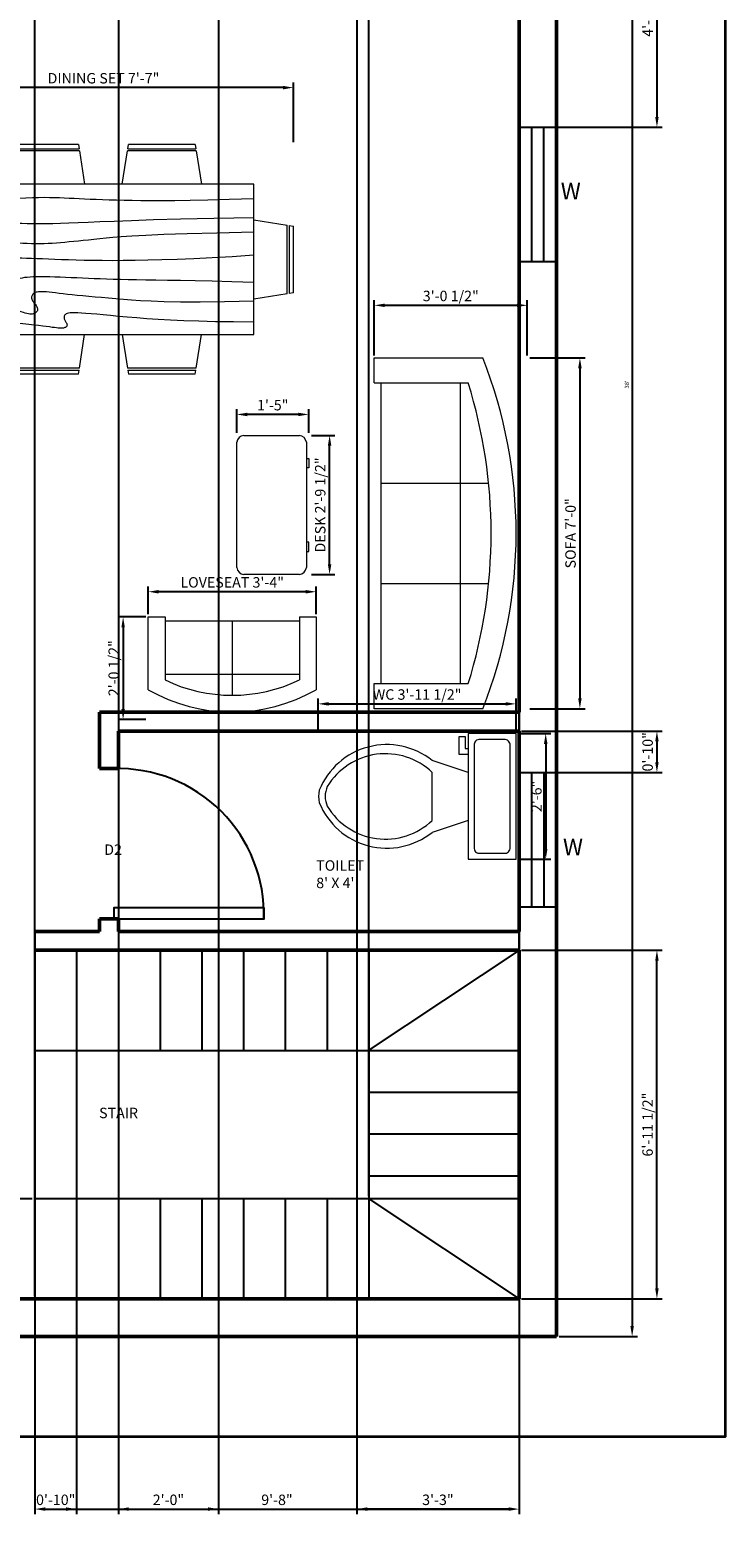
# Model space of a CAD drawing. Units: inches. Extents: x 216 to 622, y 47 to 588.
# Tile 2 of 3: x 455 to 622, y 48 to 403. Entities that reach past the tile are written whole.
import ezdxf

# ---------------------------------------------------------------- set-up
doc = ezdxf.new("R2010")
doc.units = ezdxf.units.IN
for name, color, linetype, lineweight in [('A-ANNO-TTLB', 7, 'Continuous', 35), ('A-AREA-IDEN', 7, 'Continuous', 18), ('A-DOOR', 3, 'Continuous', 25), ('A-FLOR-FIXT', 9, 'Continuous', 18), ('A-FLOR-STRS', 7, 'Continuous', 25), ('A-FURN', 8, 'Continuous', 18), ('A-GLAZ', 4, 'Continuous', 25), ('A-WALL', 7, 'Continuous', 50), ('Dimensions', 1, 'Continuous', 18), ('Text', 6, 'Continuous', 18)]:
    doc.layers.add(name, color=color, linetype=linetype, lineweight=lineweight)
doc.styles.get("Standard").update_dxf_attribs({"font": 'arial.ttf'})
doc.dimstyles.new('ISO-25', dxfattribs={"dimtxt": 2.5, "dimasz": 2.5, "dimexe": 1.25, "dimexo": 0.625, "dimtad": 1, "dimtxsty": 'Standard', "dimcen": 2.5, "dimadec": 0, "dimazin": 0, "dimtfac": 1, "dimtmove": 0, "dimatfit": 3, "dimfxl": 1, "dimarcsym": 0})

# ---------------------------------------------------------------- blocks, each defined once
blk = doc.blocks.new('Sofa - Roundback Loveseat 5 ft.')
for p, q in [((0, -32.44198), (0, -5.99998)), ((-24, -33.99998), (-24, -11.46958)), ((-23.9998, -13.38178), (23.99986, -13.38178)), ((24.00004, -33.99998), (24.00004, -11.46958)), ((-24, -32.44198), (24.00004, -32.44198))]:
    blk.add_line(p, q)
for points in [[(-24, -33.99998), (-30, -33.99998), (-30, -7.99998)], [(30.00004, -7.99998), (30.00004, -33.99998), (24.00004, -33.99998)]]:
    blk.add_lwpolyline(points)
for centre, radius, start, end in [((0, -60.24998), 60.24998, 60.13715, 119.8628), ((0, -61.38438), 55.38444, 64.32083, 115.6792)]:
    blk.add_arc(centre, radius, start, end)
blk = doc.blocks.new('Desk - 30 x 60 in.')
for p, q in [((-26.999995, 0), (26.999995, 0)), ((-29.999995, -27), (-29.999995, -3)), ((29.999995, -3), (29.999995, -27)), ((26.999995, -30), (-26.999995, -30)), ((-20.000005, -30), (-20.000005, -31)), ((-20.000005, -31), (-16.000005, -31)), ((-16.000005, -31), (-16.000005, -30)), ((15.999995, -31), (15.999995, -30)), ((19.999995, -31), (15.999995, -31)), ((19.999995, -30), (19.999995, -31))]:
    blk.add_line(p, q)
for centre, start, end in [((-26.499995, -3.5), 98.1301, 171.8699), ((26.499995, -3.5), 8.130102, 81.8699), ((-26.499995, -26.5), 188.1301, 261.8699), ((26.499995, -26.5), 278.1301, 351.8699)]:
    blk.add_arc(centre, 3.535534, start, end)
blk = doc.blocks.new('Dining Set - 36 x 72 in.')
for p, q in [((-22.2343, 26.00059), (-23.4847, 17.99762)), ((-22.2304, 26), (-5.7608, 26)), ((-22, 27.5), (-22.1562, 26.50042)), ((-5.8416, 26.5), (-22.1534, 26.5)), ((-22, 27.5), (-6, 27.5)), ((-5.8437, 26.49966), (-6, 27.5)), ((-4.5152, 17.99762), (-5.7655, 25.99926)), ((5.7657, 26.00059), (4.5153, 17.99762)), ((5.7696, 26), (22.2392, 26)), ((6, 27.5), (5.8438, 26.50042)), ((22.1584, 26.5), (5.8466, 26.5)), ((6, 27.5), (22, 27.5)), ((22.1563, 26.49966), (22, 27.5)), ((23.4848, 17.99762), (22.2345, 25.99926)), ((36, 18), (-36, 18)), ((-36, 18), (-36, -18)), ((36, -18), (36, 18)), ((-45.5, 8), (-44.5004, 8.15617)), ((-45.5, 8), (-45.5, -8)), ((-44.5, -8.15843), (-44.5, 8.15338)), ((-44.0006, 8.23428), (-35.9976, 9.48474)), ((-44, 8.23041), (-44, -8.23915)), ((44.0006, 8.23428), (35.9976, 9.48474)), ((44, 8.23041), (44, -8.23915)), ((44.5, -8.15843), (44.5, 8.15338)), ((45.5, 8), (44.5005, 8.15617)), ((45.5, 8), (45.5, -8)), ((-44.4997, -8.15631), (-45.5, -8)), ((-35.9976, -9.48476), (-43.9993, -8.2345)), ((35.9976, -9.48476), (43.9993, -8.2345)), ((44.4997, -8.15631), (45.5, -8)), ((-36, -18), (36, -18)), ((-22.2343, -26.0006), (-23.4847, -17.99762)), ((-4.5152, -17.99762), (-5.7655, -25.99928)), ((5.7657, -26.0006), (4.5153, -17.99762)), ((23.4848, -17.99762), (22.2345, -25.99928)), ((-22.2304, -26), (-5.7608, -26)), ((-22, -27.5), (-22.1562, -26.50044)), ((-5.8416, -26.5), (-22.1534, -26.5)), ((-22, -27.5), (-6, -27.5)), ((-5.8437, -26.49967), (-6, -27.5)), ((5.7696, -26), (22.2392, -26)), ((6, -27.5), (5.8438, -26.50044)), ((22.1584, -26.5), (5.8466, -26.5)), ((6, -27.5), (22, -27.5)), ((22.1563, -26.49967), (22, -27.5))]:
    blk.add_line(p, q)
for points in [[(-36, 15), (-31.1772, 14.97754), (-26.8079, 14.91406), (-22.8538, 14.81543), (-19.276, 14.6875), (-16.0362, 14.53613), (-13.0957, 14.36718), (-10.4159, 14.18652), (-7.9583, 14), (-5.6904, 13.81315), (-3.6035, 13.63021), (-1.6954, 13.45508), (0.0365, 13.29166), (1.5945, 13.14388), (2.9811, 13.01562), (4.1988, 12.9108), (5.25, 12.83333), (6.1393, 12.78613), (6.8802, 12.76823), (7.4883, 12.77767), (7.9792, 12.8125), (8.3685, 12.87077), (8.6719, 12.95052), (8.9049, 13.0498), (9.0833, 13.16666), (9.2205, 13.29899), (9.3216, 13.44401), (9.3895, 13.59879), (9.4271, 13.76041), (9.4373, 13.92594), (9.4232, 14.09245), (9.3875, 14.257), (9.3333, 14.41666), (9.2638, 14.56917), (9.1836, 14.71484), (9.0975, 14.85465), (9.0104, 14.98958), (8.9272, 15.1206), (8.8529, 15.2487), (8.7922, 15.37483), (8.75, 15.5), (8.7305, 15.62467), (8.7344, 15.74739), (8.7617, 15.86621), (8.8125, 15.97916), (8.8867, 16.08431), (8.9844, 16.17968), (9.1055, 16.26334), (9.25, 16.33333), (9.4189, 16.38802), (9.6172, 16.42708), (9.8506, 16.45052), (10.125, 16.45833), (10.4463, 16.45052), (10.8203, 16.42708), (11.2529, 16.38802), (11.75, 16.33333), (12.3184, 16.26318), (12.9694, 16.17838), (13.7151, 16.07991), (14.5677, 15.96875), (15.5395, 15.84586), (16.6426, 15.71224), (17.8893, 15.56884), (19.2917, 15.41666), (20.859, 15.25667), (22.5879, 15.08984), (24.4721, 14.91715), (26.5052, 14.73958), (28.6809, 14.5581), (30.9929, 14.3737), (33.4347, 14.18733), (36, 14)], [(-36, 10), (-28.9766, 10.14274), (-23.1725, 10.20442), (-18.4241, 10.19775), (-14.5677, 10.13541), (-11.4399, 10.03011), (-8.877, 9.89453), (-6.7154, 9.74137), (-4.7917, 9.58333), (-2.9698, 9.43082), (-1.2246, 9.28515), (0.4415, 9.14534), (2.026, 9.01041), (3.5266, 8.87939), (4.9408, 8.7513), (6.266, 8.62516), (7.5, 8.5), (8.6411, 8.37549), (9.6914, 8.2539), (10.6538, 8.13818), (11.5312, 8.03125), (12.3267, 7.93603), (13.043, 7.85547), (13.6831, 7.79248), (14.25, 7.75), (14.7471, 7.7303), (15.1797, 7.73307), (15.5537, 7.75732), (15.875, 7.80208), (16.1494, 7.86637), (16.3828, 7.94922), (16.5811, 8.04964), (16.75, 8.16666), (16.8944, 8.29915), (17.0143, 8.44531), (17.1089, 8.60319), (17.1771, 8.77083), (17.218, 8.94629), (17.2305, 9.1276), (17.2137, 9.31282), (17.1667, 9.5), (17.0895, 9.6875), (16.987, 9.875), (16.8649, 10.0625), (16.7292, 10.25), (16.5856, 10.4375), (16.4401, 10.625), (16.2985, 10.8125), (16.1667, 11), (16.05, 11.18733), (15.9518, 11.3737), (15.8752, 11.5581), (15.8229, 11.73958), (15.798, 11.91715), (15.8034, 12.08984), (15.842, 12.25667), (15.9167, 12.41666), (16.0295, 12.56836), (16.1784, 12.70833), (16.3605, 12.83268), (16.5729, 12.9375), (16.8127, 13.01888), (17.0768, 13.07291), (17.3625, 13.0957), (17.6667, 13.08333), (17.9894, 13.03312), (18.3418, 12.94726), (18.7382, 12.82918), (19.1927, 12.68229), (19.7195, 12.51001), (20.3327, 12.31575), (21.0465, 12.10294), (21.875, 11.875), (22.8357, 11.63354), (23.959, 11.37304), (25.2786, 11.08618), (26.8282, 10.76562), (28.6414, 10.40405), (30.752, 9.99414), (33.1936, 9.52856), (36, 9)], [(-36, 5.5), (-30.7157, 5.3348), (-26.069, 5.20963), (-21.9946, 5.11767), (-18.4271, 5.05208), (-15.3009, 5.00602), (-12.5508, 4.97265), (-10.1112, 4.94515), (-7.9167, 4.91666), (-5.909, 4.88167), (-4.0586, 4.83984), (-2.3429, 4.79215), (-0.7396, 4.73958), (0.7739, 4.6831), (2.22, 4.6237), (3.6213, 4.56233), (5, 4.5), (6.373, 4.43782), (7.7344, 4.3776), (9.0723, 4.32129), (10.375, 4.27083), (11.6309, 4.22819), (12.8281, 4.19531), (13.9551, 4.17415), (15, 4.16666), (15.954, 4.17448), (16.819, 4.19791), (17.6001, 4.23698), (18.3021, 4.29166), (18.9299, 4.36198), (19.4883, 4.44791), (19.9823, 4.54948), (20.4167, 4.66666), (20.7969, 4.79899), (21.1302, 4.94401), (21.4245, 5.09879), (21.6875, 5.26041), (21.9271, 5.42594), (22.1511, 5.59245), (22.3672, 5.757), (22.5834, 5.91666), (22.8065, 6.06868), (23.0404, 6.21093), (23.2879, 6.34147), (23.5521, 6.45833), (23.8358, 6.55957), (24.142, 6.64323), (24.4735, 6.70735), (24.8334, 6.75), (25.2235, 6.76969), (25.642, 6.76692), (26.0858, 6.74267), (26.5521, 6.69791), (27.0379, 6.63362), (27.5404, 6.55078), (28.0565, 6.45036), (28.5834, 6.33333), (29.1242, 6.19987), (29.7071, 6.04687), (30.3661, 5.87044), (31.1354, 5.66666), (32.0493, 5.43164), (33.142, 5.16146), (34.4475, 4.85221), (36, 4.5)], [(-36, -1), (-30.7915, -0.6591), (-26.0195, -0.38216), (-21.6519, -0.16284), (-17.6563, 0.00521), (-14.0005, 0.12833), (-10.6523, 0.21289), (-7.5796, 0.26522), (-4.75, 0.29166), (-2.134, 0.29793), (0.2878, 0.28711), (2.5317, 0.26163), (4.6146, 0.22396), (6.5529, 0.17651), (8.3633, 0.12174), (10.0623, 0.06209), (11.6667, 0), (13.1899, -0.06201), (14.6341, -0.1211), (15.9982, -0.17432), (17.2813, -0.21875), (18.4823, -0.25147), (19.6003, -0.26953), (20.6343, -0.27002), (21.5834, -0.25), (22.4481, -0.20768), (23.2357, -0.14584), (23.9549, -0.06836), (24.6146, 0.02083), (25.2235, 0.11784), (25.7904, 0.21875), (26.3241, 0.31966), (26.8334, 0.41666), (27.3265, 0.50618), (27.8099, 0.58593), (28.2894, 0.65397), (28.7709, 0.70833), (29.2601, 0.74707), (29.763, 0.76823), (30.2855, 0.76985), (30.8334, 0.75), (31.4088, 0.70784), (31.9994, 0.64713), (32.589, 0.57275), (33.1615, 0.48958), (33.7008, 0.4025), (34.1908, 0.3164), (34.6153, 0.23616), (34.9584, 0.16666), (35.2099, 0.11165), (35.3848, 0.07031), (35.504, 0.04069), (35.5886, 0.02083), (35.6594, 0.00879), (35.7377, 0.0026), (35.8442, 0.00032), (36, 0)], [(-36, -6.5), (-27.1843, -6.31267), (-20.084, -6.1263), (-14.469, -5.9419), (-10.1094, -5.76042), (-6.7752, -5.58285), (-4.2363, -5.41016), (-2.2629, -5.24333), (-0.625, -5.08334), (0.8708, -4.93099), (2.2715, -4.78646), (3.5872, -4.64974), (4.8281, -4.52084), (6.0046, -4.39974), (7.127, -4.28646), (8.2053, -4.18099), (9.25, -4.08334), (10.2705, -3.99382), (11.2734, -3.91407), (12.2647, -3.84603), (13.25, -3.79167), (14.2354, -3.75293), (15.2266, -3.73177), (16.2295, -3.73015), (17.25, -3.75), (18.2912, -3.79248), (19.3451, -3.85547), (20.4009, -3.93604), (21.4479, -4.03125), (22.4754, -4.13819), (23.4727, -4.25391), (24.4289, -4.37549), (25.3334, -4.5), (26.1785, -4.62492), (26.9694, -4.74935), (27.7145, -4.87281), (28.4219, -4.99479), (29.1, -5.11483), (29.7572, -5.23242), (30.4016, -5.34709), (31.0417, -5.45834), (31.6837, -5.56437), (32.3262, -5.65821), (32.9658, -5.73153), (33.599, -5.77604), (34.2224, -5.78345), (34.8327, -5.74545), (35.4264, -5.65373), (36, -5.5)], [(-36, -10), (-26.4022, -9.81299), (-18.4675, -9.62891), (-11.9839, -9.45069), (-6.7396, -9.28125), (-2.5226, -9.12354), (0.8789, -8.98047), (3.6769, -8.85498), (6.0833, -8.75), (8.2767, -8.66765), (10.3021, -8.60677), (12.1712, -8.56543), (13.8958, -8.54167), (15.4876, -8.53353), (16.9583, -8.53907), (18.3197, -8.55632), (19.5834, -8.58334), (20.7616, -8.61841), (21.8685, -8.66081), (22.9188, -8.71004), (23.9271, -8.76563), (24.9081, -8.82707), (25.8763, -8.89388), (26.8465, -8.96558), (27.8334, -9.04167), (28.8474, -9.12118), (29.8828, -9.20117), (30.93, -9.27824), (31.9792, -9.34896), (33.0205, -9.40991), (34.0443, -9.45768), (35.0407, -9.48885), (36, -9.5)], [(-36, -14.5), (-30.0881, -14.33513), (-25.0332, -14.21224), (-20.7312, -14.12647), (-17.0781, -14.07292), (-13.97, -14.04671), (-11.3027, -14.04297), (-8.9724, -14.05681), (-6.875, -14.08334), (-4.9224, -14.11833), (-3.0905, -14.16016), (-1.3709, -14.20785), (0.2448, -14.26042), (1.7647, -14.3169), (3.1973, -14.3763), (4.5507, -14.43767), (5.8333, -14.5), (7.0554, -14.5621), (8.235, -14.62175), (9.3922, -14.67652), (10.5469, -14.72396), (11.7192, -14.76164), (12.929, -14.78711), (14.1965, -14.79794), (15.5417, -14.79167), (16.9933, -14.76424), (18.6152, -14.70508), (20.4804, -14.60197), (22.6615, -14.44271), (25.2312, -14.21509), (28.2624, -13.9069), (31.8277, -13.50594), (36, -13)]]:
    blk.add_lwpolyline(points)
blk = doc.blocks.new('Toilet - top')
for p, q in [((9.5, -6), (9.5, -2)), ((-10, -8.5), (-8, -8.5)), ((-10, -9.5), (-10, -8.5)), ((-7, -9.5), (-10, -9.5)), ((-8, -8.5), (-8, -8)), ((-7, -8), (-7, -9.5)), ((-4, -8), (-6, -14)), ((4, -8), (6, -14)), ((4, -14), (-4, -14))]:
    blk.add_line(p, q)
blk.add_lwpolyline([(10.5, -8), (10.5, 0), (-10.5, 0), (-10.5, -8)], close=True)
for points in [[(-9.5, -2), (-9.5, -6)], [(8.5, -1), (-8.5, -1)], [(-8.5, -7), (8.5, -7)]]:
    blk.add_lwpolyline(points)
for centre, radius, start, end in [((-8.62, -1.88), 0.884, 81.8699, 188.1301), ((8.62, -1.88), 0.884, 351.8699, 98.1301), ((-8.62, -6.12), 0.884, 171.8699, 278.1301), ((8.62, -6.12), 0.884, 261.8699, 8.1301), ((3.52, -21.58), 12.17, 141.4691, 247.9714), ((4.2, -21.82), 11.33, 136.3677, 238.9468), ((-3.52, -21.58), 12.17, 292.0284, 38.5307), ((-4.2, -21.82), 11.33, 301.053, 43.6321), ((0, -27.88), 4, 245.7318, 294.2682), ((0, -29), 4, 254.8605, 285.1395)]:
    blk.add_arc(centre, radius, start, end)
blk = doc.blocks.new('Sofa - Roundback 7 ft.')
for p, q in [((-12.00002, -32.4421), (-12.00003, -6.5971)), ((11.99997, -32.4421), (11.99998, -6.5971)), ((-36.000027, -34), (-36.000027, -11.4696)), ((-35.999844, -13.3819), (35.9998, -13.3819)), ((35.99998, -34), (35.99998, -11.4696)), ((-36.000027, -32.4421), (35.99998, -32.4421))]:
    blk.add_line(p, q)
for points in [[(-36.000027, -34), (-42.000027, -34), (-42.000027, -8)], [(41.99998, -8), (41.99998, -34), (35.99998, -34)]]:
    blk.add_lwpolyline(points)
for centre, radius, start, end in [((0, -114.25), 114.25, 68.43141, 111.5686), ((-0.00001, -127.1968), 121.1968, 72.72033, 107.2797)]:
    blk.add_arc(centre, radius, start, end)
blk = doc.blocks.new('*D12')
at = {"layer": 'Defpoints', "color": 0, "transparency": 16777216}
for p in [(581.54, 546.47), (581.54, 90.47), (599.64, 90.47)]:
    blk.add_point(p, dxfattribs=at)
at = {"layer": 'Dimensions', "color": 0, "lineweight": -2, "transparency": 16777216}
for p, q in [((582.16, 546.47), (600.89, 546.47)), ((599.64, 543.97), (599.64, 92.97)), ((582.16, 90.47), (600.89, 90.47))]:
    blk.add_line(p, q, dxfattribs=at)
at = {"layer": 'Dimensions', "color": 0, "transparency": 16777216}
for points in [[(599.22, 543.97), (600.05, 543.97), (599.64, 546.47)], [(599.22, 92.97), (600.05, 92.97), (599.64, 90.47)]]:
    blk.add_solid(points, dxfattribs=at)
at = {"layer": 'Dimensions', "color": 0, "transparency": 16777216, "insert": (598.5, 318.47), "char_height": 1, "attachment_point": 5, "rotation": 90}
blk.add_mtext("38'", dxfattribs=at)
blk = doc.blocks.new('WINDOW-W-PLAN')
for p, q in [((0, 0), (0, 32.22)), ((0, 32.22), (9, 32.22)), ((3, 32.22), (3, 0)), ((6, 0), (6, 32.22)), ((9, 32.22), (9, 0)), ((9, 0), (0, 0))]:
    blk.add_line(p, q)
blk = doc.blocks.new('DOOR-PANEL-36IN-NOM')
blk.add_lwpolyline([(35.86, 2.79), (35.86, 0), (0, 0), (0, 2.79)], close=True)
blk = doc.blocks.new('*D29')
at = {"layer": 'Defpoints', "color": 0, "transparency": 16777216}
for p in [(571.82, 241.97), (524.42, 234.87), (571.82, 234.87)]:
    blk.add_point(p, dxfattribs=at)
at = {"layer": 'Dimensions', "color": 0, "lineweight": -2, "transparency": 16777216}
for p, q in [((524.42, 235.49), (524.42, 243.22)), ((526.92, 241.97), (569.32, 241.97)), ((571.82, 235.49), (571.82, 243.22))]:
    blk.add_line(p, q, dxfattribs=at)
at = {"layer": 'Dimensions', "color": 0, "transparency": 16777216}
for points in [[(526.92, 242.39), (526.92, 241.56), (524.42, 241.97)], [(569.32, 242.39), (569.32, 241.56), (571.82, 241.97)]]:
    blk.add_solid(points, dxfattribs=at)
at = {"layer": 'Dimensions', "color": 0, "transparency": 16777216, "insert": (548.12, 243.89), "char_height": 2.5, "attachment_point": 5}
blk.add_mtext('WC 3\'-11 1/2"', dxfattribs=at)
blk = doc.blocks.new('*D30')
at = {"layer": 'Defpoints', "color": 0, "transparency": 16777216}
for p in [(571.82, 234.87), (571.82, 204.75), (578.93, 204.75)]:
    blk.add_point(p, dxfattribs=at)
at = {"layer": 'Dimensions', "color": 0, "lineweight": -2, "transparency": 16777216}
for p, q in [((572.45, 234.87), (580.18, 234.87)), ((578.93, 232.37), (578.93, 207.25)), ((572.45, 204.75), (580.18, 204.75))]:
    blk.add_line(p, q, dxfattribs=at)
at = {"layer": 'Dimensions', "color": 0, "transparency": 16777216}
for points in [[(578.51, 232.37), (579.35, 232.37), (578.93, 234.87)], [(578.51, 207.25), (579.35, 207.25), (578.93, 204.75)]]:
    blk.add_solid(points, dxfattribs=at)
at = {"layer": 'Dimensions', "color": 0, "transparency": 16777216, "insert": (577.03, 219.81), "char_height": 2.5, "attachment_point": 5, "rotation": 90}
blk.add_mtext('2\'-6"', dxfattribs=at)
blk = doc.blocks.new('*D37')
at = {"layer": 'Defpoints', "color": 0, "transparency": 16777216}
for p in [(427.48, 389.56), (427.48, 375.91), (518.48, 375.91)]:
    blk.add_point(p, dxfattribs=at)
at = {"layer": 'Dimensions', "color": 0, "lineweight": -2, "transparency": 16777216}
for p, q in [((427.48, 376.53), (427.48, 390.81)), ((515.98, 389.56), (429.98, 389.56)), ((518.48, 376.53), (518.48, 390.81))]:
    blk.add_line(p, q, dxfattribs=at)
at = {"layer": 'Dimensions', "color": 0, "transparency": 16777216}
for points in [[(429.98, 389.98), (429.98, 389.14), (427.48, 389.56)], [(515.98, 389.98), (515.98, 389.14), (518.48, 389.56)]]:
    blk.add_solid(points, dxfattribs=at)
at = {"layer": 'Dimensions', "color": 0, "transparency": 16777216, "insert": (472.98, 391.48), "char_height": 2.5, "attachment_point": 5}
blk.add_mtext('DINING SET 7\'-7"', dxfattribs=at)
blk = doc.blocks.new('*D39')
at = {"layer": 'Defpoints', "color": 0, "transparency": 16777216}
for p in [(574.52, 324.82), (574.52, 240.82), (587.12, 240.82)]:
    blk.add_point(p, dxfattribs=at)
at = {"layer": 'Dimensions', "color": 0, "lineweight": -2, "transparency": 16777216}
for p, q in [((575.15, 324.82), (588.37, 324.82)), ((587.12, 322.32), (587.12, 243.32)), ((575.15, 240.82), (588.37, 240.82))]:
    blk.add_line(p, q, dxfattribs=at)
at = {"layer": 'Dimensions', "color": 0, "transparency": 16777216}
for points in [[(586.7, 322.32), (587.54, 322.32), (587.12, 324.82)], [(586.7, 243.32), (587.54, 243.32), (587.12, 240.82)]]:
    blk.add_solid(points, dxfattribs=at)
at = {"layer": 'Dimensions', "color": 0, "transparency": 16777216, "insert": (585.2, 282.82), "char_height": 2.5, "attachment_point": 5, "rotation": 90}
blk.add_mtext('SOFA 7\'-0"', dxfattribs=at)
blk = doc.blocks.new('*D40')
at = {"layer": 'Defpoints', "color": 0, "transparency": 16777216}
for p in [(574.52, 337.42), (537.85, 324.82), (574.52, 324.82)]:
    blk.add_point(p, dxfattribs=at)
at = {"layer": 'Dimensions', "color": 0, "lineweight": -2, "transparency": 16777216}
for p, q in [((537.85, 325.44), (537.85, 338.67)), ((574.52, 325.44), (574.52, 338.67)), ((540.35, 337.42), (572.02, 337.42))]:
    blk.add_line(p, q, dxfattribs=at)
at = {"layer": 'Dimensions', "color": 0, "transparency": 16777216}
for points in [[(540.35, 337.83), (540.35, 337), (537.85, 337.42)], [(572.02, 337.83), (572.02, 337), (574.52, 337.42)]]:
    blk.add_solid(points, dxfattribs=at)
at = {"layer": 'Dimensions', "color": 0, "transparency": 16777216, "insert": (556.19, 339.34), "char_height": 2.5, "attachment_point": 5}
blk.add_mtext('3\'-0 1/2"', dxfattribs=at)
blk = doc.blocks.new('*D41')
at = {"layer": 'Defpoints', "color": 0, "transparency": 16777216}
for p in [(522.15, 306.28), (527.15, 306.28), (522.15, 272.93)]:
    blk.add_point(p, dxfattribs=at)
at = {"layer": 'Dimensions', "color": 0, "lineweight": -2, "transparency": 16777216}
for p, q in [((522.78, 306.28), (528.4, 306.28)), ((527.15, 275.43), (527.15, 303.78)), ((522.78, 272.93), (528.4, 272.93))]:
    blk.add_line(p, q, dxfattribs=at)
at = {"layer": 'Dimensions', "color": 0, "transparency": 16777216}
for points in [[(526.74, 303.78), (527.57, 303.78), (527.15, 306.28)], [(526.74, 275.43), (527.57, 275.43), (527.15, 272.93)]]:
    blk.add_solid(points, dxfattribs=at)
at = {"layer": 'Dimensions', "color": 0, "transparency": 16777216, "insert": (525.24, 289.61), "char_height": 2.5, "attachment_point": 5, "rotation": 90}
blk.add_mtext('DESK 2\'-9 1/2"', dxfattribs=at)
blk = doc.blocks.new('*D42')
at = {"layer": 'Defpoints', "color": 0, "transparency": 16777216}
for p in [(504.92, 311.29), (504.92, 306.28), (522.15, 306.28)]:
    blk.add_point(p, dxfattribs=at)
at = {"layer": 'Dimensions', "color": 0, "lineweight": -2, "transparency": 16777216}
for p, q in [((504.92, 306.91), (504.92, 312.54)), ((519.65, 311.29), (507.42, 311.29)), ((522.15, 306.91), (522.15, 312.54))]:
    blk.add_line(p, q, dxfattribs=at)
at = {"layer": 'Dimensions', "color": 0, "transparency": 16777216}
for points in [[(507.42, 311.7), (507.42, 310.87), (504.92, 311.29)], [(519.65, 311.7), (519.65, 310.87), (522.15, 311.29)]]:
    blk.add_solid(points, dxfattribs=at)
at = {"layer": 'Dimensions', "color": 0, "transparency": 16777216, "insert": (513.53, 313.19), "char_height": 2.5, "attachment_point": 5}
blk.add_mtext('1\'-5"', dxfattribs=at)
blk = doc.blocks.new('*D43')
at = {"layer": 'Defpoints', "color": 0, "transparency": 16777216}
for p in [(483.71, 268.83), (483.71, 262.8), (523.93, 262.8)]:
    blk.add_point(p, dxfattribs=at)
at = {"layer": 'Dimensions', "color": 0, "lineweight": -2, "transparency": 16777216}
for p, q in [((483.71, 263.42), (483.71, 270.08)), ((521.43, 268.83), (486.21, 268.83)), ((523.93, 263.42), (523.93, 270.08))]:
    blk.add_line(p, q, dxfattribs=at)
at = {"layer": 'Dimensions', "color": 0, "transparency": 16777216}
for points in [[(486.21, 269.24), (486.21, 268.41), (483.71, 268.83)], [(521.43, 269.24), (521.43, 268.41), (523.93, 268.83)]]:
    blk.add_solid(points, dxfattribs=at)
at = {"layer": 'Dimensions', "color": 0, "transparency": 16777216, "insert": (503.82, 270.75), "char_height": 2.5, "attachment_point": 5}
blk.add_mtext('LOVESEAT 3\'-4"', dxfattribs=at)
blk = doc.blocks.new('*D44')
at = {"layer": 'Defpoints', "color": 0, "transparency": 16777216}
for p in [(483.71, 262.8), (477.68, 238.22), (483.71, 238.22)]:
    blk.add_point(p, dxfattribs=at)
at = {"layer": 'Dimensions', "color": 0, "lineweight": -2, "transparency": 16777216}
for p, q in [((483.09, 262.8), (476.43, 262.8)), ((477.68, 260.3), (477.68, 240.72)), ((483.09, 238.22), (476.43, 238.22))]:
    blk.add_line(p, q, dxfattribs=at)
at = {"layer": 'Dimensions', "color": 0, "transparency": 16777216}
for points in [[(477.27, 260.3), (478.1, 260.3), (477.68, 262.8)], [(477.27, 240.72), (478.1, 240.72), (477.68, 238.22)]]:
    blk.add_solid(points, dxfattribs=at)
at = {"layer": 'Dimensions', "color": 0, "transparency": 16777216, "insert": (475.76, 250.51), "char_height": 2.5, "attachment_point": 5, "rotation": 90}
blk.add_mtext('2\'-0 1/2"', dxfattribs=at)
blk = doc.blocks.new('*D47')
at = {"layer": 'Defpoints', "color": 0, "transparency": 16777216}
for p in [(533.67, 537.45), (572.54, 537.47), (533.67, 49.13)]:
    blk.add_point(p, dxfattribs=at)
at = {"layer": 'Dimensions', "color": 0, "lineweight": -2, "transparency": 16777216}
for p, q in [((533.67, 536.83), (533.67, 47.88)), ((572.54, 536.84), (572.54, 47.88)), ((570.04, 49.13), (536.17, 49.13))]:
    blk.add_line(p, q, dxfattribs=at)
at = {"layer": 'Dimensions', "color": 0, "transparency": 16777216}
for points in [[(536.17, 49.55), (536.17, 48.71), (533.67, 49.13)], [(570.04, 49.55), (570.04, 48.71), (572.54, 49.13)]]:
    blk.add_solid(points, dxfattribs=at)
at = {"layer": 'Dimensions', "color": 0, "transparency": 16777216, "insert": (553.1, 51.03), "char_height": 2.5, "attachment_point": 5}
blk.add_mtext('3\'-3"', dxfattribs=at)
blk = doc.blocks.new('*D52')
at = {"layer": 'Defpoints', "color": 0, "transparency": 16777216}
for p in [(572.54, 235.47), (572.55, 225.51), (605.57, 225.51)]:
    blk.add_point(p, dxfattribs=at)
at = {"layer": 'Dimensions', "color": 0, "lineweight": -2, "transparency": 16777216}
for p, q in [((573.16, 235.47), (606.82, 235.47)), ((605.57, 232.97), (605.57, 228.01)), ((573.18, 225.51), (606.82, 225.51))]:
    blk.add_line(p, q, dxfattribs=at)
at = {"layer": 'Dimensions', "color": 0, "transparency": 16777216}
for points in [[(605.16, 232.97), (605.99, 232.97), (605.57, 235.47)], [(605.16, 228.01), (605.99, 228.01), (605.57, 225.51)]]:
    blk.add_solid(points, dxfattribs=at)
at = {"layer": 'Dimensions', "color": 0, "transparency": 16777216, "insert": (603.67, 230.49), "char_height": 2.5, "attachment_point": 5, "rotation": 90}
blk.add_mtext('0\'-10"', dxfattribs=at)
blk = doc.blocks.new('*D53')
at = {"layer": 'Defpoints', "color": 0, "transparency": 16777216}
for p in [(572.54, 430.97), (572.51, 380.05), (605.57, 380.05)]:
    blk.add_point(p, dxfattribs=at)
at = {"layer": 'Dimensions', "color": 0, "lineweight": -2, "transparency": 16777216}
for p, q in [((573.16, 430.97), (606.82, 430.97)), ((605.57, 428.47), (605.57, 382.55)), ((573.13, 380.05), (606.82, 380.05))]:
    blk.add_line(p, q, dxfattribs=at)
at = {"layer": 'Dimensions', "color": 0, "transparency": 16777216}
for points in [[(605.16, 428.47), (605.99, 428.47), (605.57, 430.97)], [(605.16, 382.55), (605.99, 382.55), (605.57, 380.05)]]:
    blk.add_solid(points, dxfattribs=at)
at = {"layer": 'Dimensions', "color": 0, "transparency": 16777216, "insert": (603.67, 405.51), "char_height": 2.5, "attachment_point": 5, "rotation": 90}
blk.add_mtext('4\'-3"', dxfattribs=at)
blk = doc.blocks.new('*D57')
at = {"layer": 'Defpoints', "color": 0, "transparency": 16777216}
for p in [(456.54, 99.47), (572.54, 99.47), (572.54, 49.13)]:
    blk.add_point(p, dxfattribs=at)
at = {"layer": 'Dimensions', "color": 0, "lineweight": -2, "transparency": 16777216}
for p, q in [((456.54, 98.84), (456.54, 47.88)), ((572.54, 98.84), (572.54, 47.88)), ((459.04, 49.13), (570.04, 49.13))]:
    blk.add_line(p, q, dxfattribs=at)
at = {"layer": 'Dimensions', "color": 0, "transparency": 16777216}
for points in [[(459.04, 49.55), (459.04, 48.71), (456.54, 49.13)], [(570.04, 49.55), (570.04, 48.71), (572.54, 49.13)]]:
    blk.add_solid(points, dxfattribs=at)
at = {"layer": 'Dimensions', "color": 0, "transparency": 16777216, "insert": (514.54, 51.03), "char_height": 2.5, "attachment_point": 5}
blk.add_mtext('9\'-8"', dxfattribs=at)
blk = doc.blocks.new('*D58')
at = {"layer": 'Defpoints', "color": 0, "transparency": 16777216}
for p in [(572.54, 182.97), (605.57, 182.97), (572.54, 99.47)]:
    blk.add_point(p, dxfattribs=at)
at = {"layer": 'Dimensions', "color": 0, "lineweight": -2, "transparency": 16777216}
for p, q in [((573.16, 182.97), (606.82, 182.97)), ((605.57, 101.97), (605.57, 180.47)), ((573.16, 99.47), (606.82, 99.47))]:
    blk.add_line(p, q, dxfattribs=at)
at = {"layer": 'Dimensions', "color": 0, "transparency": 16777216}
for points in [[(605.16, 180.47), (605.99, 180.47), (605.57, 182.97)], [(605.16, 101.97), (605.99, 101.97), (605.57, 99.47)]]:
    blk.add_solid(points, dxfattribs=at)
at = {"layer": 'Dimensions', "color": 0, "transparency": 16777216, "insert": (603.66, 141.22), "char_height": 2.5, "attachment_point": 5, "rotation": 90}
blk.add_mtext('6\'-11 1/2"', dxfattribs=at)
blk = doc.blocks.new('*D60')
at = {"layer": 'Defpoints', "color": 0, "transparency": 16777216}
for p in [(456.54, 182.97), (466.54, 182.97), (466.54, 49.13)]:
    blk.add_point(p, dxfattribs=at)
at = {"layer": 'Dimensions', "color": 0, "lineweight": -2, "transparency": 16777216}
for p, q in [((456.54, 182.34), (456.54, 47.88)), ((466.54, 182.34), (466.54, 47.88)), ((459.04, 49.13), (464.04, 49.13))]:
    blk.add_line(p, q, dxfattribs=at)
at = {"layer": 'Dimensions', "color": 0, "transparency": 16777216}
for points in [[(459.04, 49.55), (459.04, 48.71), (456.54, 49.13)], [(464.04, 49.55), (464.04, 48.71), (466.54, 49.13)]]:
    blk.add_solid(points, dxfattribs=at)
at = {"layer": 'Dimensions', "color": 0, "transparency": 16777216, "insert": (461.54, 51.03), "char_height": 2.5, "attachment_point": 5}
blk.add_mtext('0\'-10"', dxfattribs=at)
blk = doc.blocks.new('*D61')
at = {"layer": 'Defpoints', "color": 0, "transparency": 16777216}
for p in [(221.29, 123.47), (456.54, 123.47), (456.54, 99.47)]:
    blk.add_point(p, dxfattribs=at)
at = {"layer": 'Dimensions', "color": 0, "lineweight": -2, "transparency": 16777216}
for p, q in [((455.91, 123.47), (220.04, 123.47)), ((221.29, 101.97), (221.29, 120.97)), ((455.91, 99.47), (220.04, 99.47))]:
    blk.add_line(p, q, dxfattribs=at)
at = {"layer": 'Dimensions', "color": 0, "transparency": 16777216}
for points in [[(220.88, 120.97), (221.71, 120.97), (221.29, 123.47)], [(220.88, 101.97), (221.71, 101.97), (221.29, 99.47)]]:
    blk.add_solid(points, dxfattribs=at)
at = {"layer": 'Dimensions', "color": 0, "transparency": 16777216, "insert": (219.39, 111.47), "char_height": 2.5, "attachment_point": 5, "rotation": 90}
blk.add_mtext('2\'-0"', dxfattribs=at)
blk = doc.blocks.new('*D62')
at = {"layer": 'Defpoints', "color": 0, "transparency": 16777216}
for p in [(456.54, 570.49), (409.04, 99.47), (456.54, 99.47)]:
    blk.add_point(p, dxfattribs=at)
at = {"layer": 'Dimensions', "color": 0, "lineweight": -2, "transparency": 16777216}
for p, q in [((409.04, 100.09), (409.04, 571.74)), ((411.54, 570.49), (454.04, 570.49)), ((456.54, 100.09), (456.54, 571.74))]:
    blk.add_line(p, q, dxfattribs=at)
at = {"layer": 'Dimensions', "color": 0, "transparency": 16777216}
for points in [[(411.54, 570.9), (411.54, 570.07), (409.04, 570.49)], [(454.04, 570.9), (454.04, 570.07), (456.54, 570.49)]]:
    blk.add_solid(points, dxfattribs=at)
at = {"layer": 'Dimensions', "color": 0, "transparency": 16777216, "insert": (432.79, 572.4), "char_height": 2.5, "attachment_point": 5}
blk.add_mtext('3\'-11 1/2"', dxfattribs=at)
blk = doc.blocks.new('*D63')
at = {"layer": 'Defpoints', "color": 0, "transparency": 16777216}
for p in [(476.54, 430.97), (500.54, 430.97), (500.54, 49.13)]:
    blk.add_point(p, dxfattribs=at)
at = {"layer": 'Dimensions', "color": 0, "lineweight": -2, "transparency": 16777216}
for p, q in [((476.54, 430.34), (476.54, 47.88)), ((500.54, 430.34), (500.54, 47.88)), ((479.04, 49.13), (498.04, 49.13))]:
    blk.add_line(p, q, dxfattribs=at)
at = {"layer": 'Dimensions', "color": 0, "transparency": 16777216}
for points in [[(479.04, 49.55), (479.04, 48.71), (476.54, 49.13)], [(498.04, 49.55), (498.04, 48.71), (500.54, 49.13)]]:
    blk.add_solid(points, dxfattribs=at)
at = {"layer": 'Dimensions', "color": 0, "transparency": 16777216, "insert": (488.54, 51.03), "char_height": 2.5, "attachment_point": 5}
blk.add_mtext('2\'-0"', dxfattribs=at)
blk = doc.blocks.new('*D65')
at = {"layer": 'Defpoints', "color": 0, "transparency": 16777216}
for p in [(572.54, 570.49), (536.55, 123.47), (572.54, 123.47)]:
    blk.add_point(p, dxfattribs=at)
at = {"layer": 'Dimensions', "color": 0, "lineweight": -2, "transparency": 16777216}
for p, q in [((536.55, 124.09), (536.55, 571.74)), ((539.05, 570.49), (570.04, 570.49)), ((572.54, 124.09), (572.54, 571.74))]:
    blk.add_line(p, q, dxfattribs=at)
at = {"layer": 'Dimensions', "color": 0, "transparency": 16777216}
for points in [[(539.05, 570.9), (539.05, 570.07), (536.55, 570.49)], [(570.04, 570.9), (570.04, 570.07), (572.54, 570.49)]]:
    blk.add_solid(points, dxfattribs=at)
at = {"layer": 'Dimensions', "color": 0, "transparency": 16777216, "insert": (554.54, 572.39), "char_height": 2.5, "attachment_point": 5}
blk.add_mtext('3\'-0"', dxfattribs=at)

msp = doc.modelspace()

# ---------------------------------------------------------------- linework, layer by layer
at = {"layer": 'A-ANNO-TTLB'}
msp.add_lwpolyline([(217.87, 587.77), (621.96, 587.77), (621.96, 66.45), (217.87, 66.45)], close=True, dxfattribs=at)
at = {"layer": 'A-DOOR'}
msp.add_arc((476.46, 191.51), 34.96, 358.2243, 91.8217, dxfattribs=at)
at = {"layer": 'A-FLOR-STRS'}
for p, q in [((456.54, 187.47), (456.54, 99.47)), ((466.54, 182.97), (466.54, 158.97)), ((476.54, 182.97), (476.54, 158.97)), ((486.54, 182.97), (486.54, 158.97)), ((496.54, 182.97), (496.54, 158.97)), ((506.54, 182.97), (506.54, 158.97)), ((516.54, 182.97), (516.54, 158.97)), ((526.54, 182.97), (526.54, 158.97)), ((536.51, 158.93), (572.57, 182.9)), ((536.54, 182.97), (536.54, 99.47)), ((456.54, 158.97), (572.54, 158.97)), ((536.54, 148.97), (572.54, 148.97)), ((536.54, 138.97), (572.54, 138.97)), ((536.54, 128.97), (572.54, 128.97)), ((572.54, 123.47), (456.54, 123.47)), ((466.54, 123.47), (466.54, 99.47)), ((476.54, 123.47), (476.54, 99.47)), ((486.54, 123.47), (486.54, 99.47)), ((496.54, 123.47), (496.54, 99.47)), ((506.54, 123.47), (506.54, 99.47)), ((516.54, 123.47), (516.54, 99.47)), ((526.54, 123.47), (526.54, 99.47)), ((536.55, 123.47), (572.54, 99.46))]:
    msp.add_line(p, q, dxfattribs=at)
at = {"layer": 'A-WALL'}
for p, q in [((581.54, 546.47), (581.54, 90.47)), ((572.54, 430.97), (572.54, 239.97)), ((472.04, 239.97), (472.04, 226.47)), ((472.04, 239.97), (572.54, 239.97)), ((476.54, 235.47), (476.54, 226.47)), ((476.54, 235.47), (572.54, 235.47)), ((572.54, 235.47), (572.54, 187.47)), ((472.04, 226.47), (476.54, 226.47)), ((472.04, 190.47), (476.54, 190.47)), ((472.04, 190.47), (472.04, 187.47)), ((476.54, 190.47), (476.54, 187.47)), ((456.54, 187.47), (472.04, 187.47)), ((476.54, 187.47), (572.54, 187.47)), ((456.54, 182.97), (572.54, 182.97)), ((572.54, 182.97), (572.54, 99.47)), ((572.54, 99.47), (448.04, 99.47)), ((581.54, 90.47), (448.04, 90.47))]:
    msp.add_line(p, q, dxfattribs=at)

# ---------------------------------------------------------------- block references
at = {"layer": 'A-DOOR'}
msp.add_blockref('DOOR-PANEL-36IN-NOM', (475.54, 190.44), dxfattribs=at)
at = {"layer": 'A-FLOR-FIXT', "xscale": 1.434216897185852, "yscale": 1.434216897185852, "zscale": 1.434216897185852, "rotation": 270}
msp.add_blockref('Toilet - top', (571.82, 219.81), dxfattribs=at)
at = {"layer": 'A-FURN'}
for name, p, rotation in [('Dining Set - 36 x 72 in.', (472.98, 348.41), 180), ('Sofa - Roundback 7 ft.', (571.85, 282.82), 270)]:
    msp.add_blockref(name, p, dxfattribs=dict(at, rotation=rotation))
for name, p, xscale, yscale, zscale, rotation in [('Desk - 30 x 60 in.', (504.92, 289.61), 0.5558485250826334, 0.5558485250826334, 0.5558485250826334, 90), ('Sofa - Roundback Loveseat 5 ft.', (503.82, 240.01), 0.6701874561865664, 0.6701874561865664, 0.6701874561865664, 180)]:
    msp.add_blockref(name, p, dxfattribs=dict(at, xscale=xscale, yscale=yscale, zscale=zscale, rotation=rotation))
at = {"layer": 'A-GLAZ', "rotation": 180}
for p in [(581.51, 380.05), (581.55, 225.51)]:
    msp.add_blockref('WINDOW-W-PLAN', p, dxfattribs=at)

# ---------------------------------------------------------------- texts
at = {"layer": 'A-AREA-IDEN', "char_height": 2.5, "attachment_point": 1}
for s, width, insert in [("TOILET\\P8' X 4'", 19.8421, (523.95, 204.51)), ('STAIR', 24.9224, (471.93, 145.25))]:
    msp.add_mtext_dynamic_manual_height_columns(s, width=width, gutter_width=12.5, heights=[0], dxfattribs=dict(at, insert=insert))
at = {"layer": 'Text', "attachment_point": 1}
for s, width, gutter_width, insert, char_height in [('W', 20.8525, 20.07, (582.53, 366.79), 4.01), ('D2', 12.4782, 12.5, (473.16, 208.31), 2.5), ('W', 20.8525, 20.07, (583.06, 209.71), 4.01)]:
    msp.add_mtext_dynamic_manual_height_columns(s, width=width, gutter_width=gutter_width, heights=[0], dxfattribs=dict(at, insert=insert, char_height=char_height))

# ---------------------------------------------------------------- dimensions: what is measured, and where the dimension line sits
at = {"layer": 'Dimensions'}
for base, p1, p2, picture, middle in [((456.54, 570.49), (409.04, 99.47), (456.54, 99.47), '*D62', (432.79, 572.4)), ((572.54, 570.49), (536.55, 123.47), (572.54, 123.47), '*D65', (554.54, 572.39)), ((533.67, 49.13), (572.54, 537.47), (533.67, 537.45), '*D47', (553.1, 51.03)), ((500.54, 49.13), (476.54, 430.97), (500.54, 430.97), '*D63', (488.54, 51.03)), ((574.52, 337.42), (537.85, 324.82), (574.52, 324.82), '*D40', (556.19, 339.34)), ((466.54, 49.13), (456.54, 182.97), (466.54, 182.97), '*D60', (461.54, 51.03)), ((572.54, 49.13), (456.54, 99.47), (572.54, 99.47), '*D57', (514.54, 51.03))]:
    dim = msp.add_linear_dim(base=base, p1=p1, p2=p2, dimstyle='ISO-25', override={"dimdec": 1, "dimlfac": 1, "dimrnd": 0, "dimzin": 1, "dimdsep": 46, "dimlunit": 4, "dimfrac": 2}, dxfattribs=at)
    dim.commit()
    dim.dimension.update_dxf_attribs({"geometry": picture, "text_midpoint": middle})
for base, p1, p2, angle, override, picture, middle in [((599.64, 90.47), (581.54, 546.47), (581.54, 90.47), 90, {"dimtxt": 1, "dimdec": 0, "dimlunit": 3, "dimclrd": 0, "dimclre": 0, "dimclrt": 0, "dimtdec": 0}, '*D12', (598.5, 318.47)), ((605.57, 380.05), (572.54, 430.97), (572.51, 380.05), 90, {"dimdec": 1, "dimlfac": 1, "dimrnd": 0, "dimzin": 1, "dimdsep": 46, "dimlunit": 4, "dimfrac": 2}, '*D53', (603.67, 405.51)), ((504.92, 311.29), (522.15, 306.28), (504.92, 306.28), 180, {"dimdec": 1, "dimlfac": 1, "dimrnd": 0, "dimzin": 1, "dimdsep": 46, "dimlunit": 4, "dimfrac": 2}, '*D42', (513.53, 313.19)), ((477.68, 238.22), (483.71, 262.8), (483.71, 238.22), 270, {"dimdec": 1, "dimlfac": 1, "dimrnd": 0, "dimzin": 1, "dimdsep": 46, "dimlunit": 4, "dimfrac": 2}, '*D44', (475.76, 250.51)), ((578.93, 204.75), (571.82, 234.87), (571.82, 204.75), 270, {"dimdec": 1, "dimlfac": 1, "dimrnd": 0, "dimzin": 1, "dimdsep": 46, "dimlunit": 4, "dimfrac": 2}, '*D30', (577.03, 219.81)), ((605.57, 225.51), (572.54, 235.47), (572.55, 225.51), 90, {"dimdec": 1, "dimlfac": 1, "dimrnd": 0, "dimzin": 1, "dimdsep": 46, "dimlunit": 4, "dimfrac": 2}, '*D52', (603.67, 230.49)), ((605.57, 182.97), (572.54, 99.47), (572.54, 182.97), 90, {"dimdec": 1, "dimlfac": 1, "dimrnd": 0, "dimzin": 1, "dimdsep": 46, "dimlunit": 4, "dimfrac": 2}, '*D58', (603.66, 141.22)), ((221.29, 123.47), (456.54, 99.47), (456.54, 123.47), 90, {"dimdec": 1, "dimlfac": 1, "dimrnd": 0, "dimzin": 1, "dimdsep": 46, "dimlunit": 4, "dimfrac": 2}, '*D61', (219.39, 111.47))]:
    dim = msp.add_linear_dim(base=base, p1=p1, p2=p2, angle=angle, dimstyle='ISO-25', override=override, dxfattribs=at)
    dim.commit()
    dim.dimension.update_dxf_attribs({"geometry": picture, "text_midpoint": middle})
for base, p1, p2, angle, text, picture, middle in [((427.48, 389.56), (518.48, 375.91), (427.48, 375.91), 180, 'DINING SET <>', '*D37', (472.98, 391.48)), ((587.12, 240.82), (574.52, 324.82), (574.52, 240.82), 270, 'SOFA <>', '*D39', (585.2, 282.82)), ((527.1531, 306.2832), (522.1505, 272.9323), (522.1505, 306.2832), 90, 'DESK <>', '*D41', (525.2355, 289.6078)), ((483.71, 268.83), (523.93, 262.8), (483.71, 262.8), 180, 'LOVESEAT <>', '*D43', (503.82, 270.75))]:
    dim = msp.add_linear_dim(base=base, p1=p1, p2=p2, angle=angle, text=text, dimstyle='ISO-25', override={"dimdec": 1, "dimlfac": 1, "dimrnd": 0, "dimzin": 1, "dimdsep": 46, "dimlunit": 4, "dimfrac": 2}, dxfattribs=at)
    dim.commit()
    dim.dimension.update_dxf_attribs({"geometry": picture, "text_midpoint": middle})
dim = msp.add_linear_dim(base=(571.82, 241.97), p1=(524.42, 234.87), p2=(571.82, 234.87), text='WC <>', dimstyle='ISO-25', override={"dimdec": 1, "dimlfac": 1, "dimrnd": 0, "dimzin": 1, "dimdsep": 46, "dimlunit": 4, "dimfrac": 2}, dxfattribs=at)
dim.commit()
dim.dimension.update_dxf_attribs({"geometry": '*D29', "text_midpoint": (548.12, 243.89)})

doc.saveas('drawing.dxf')
